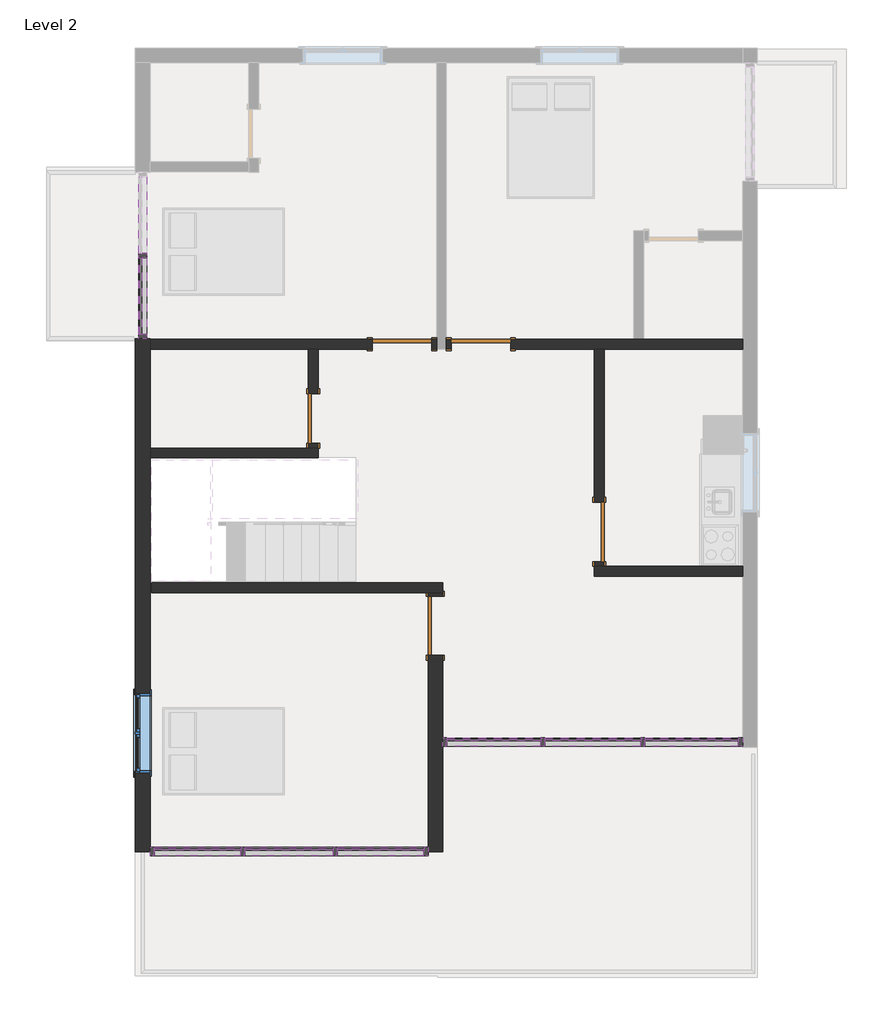
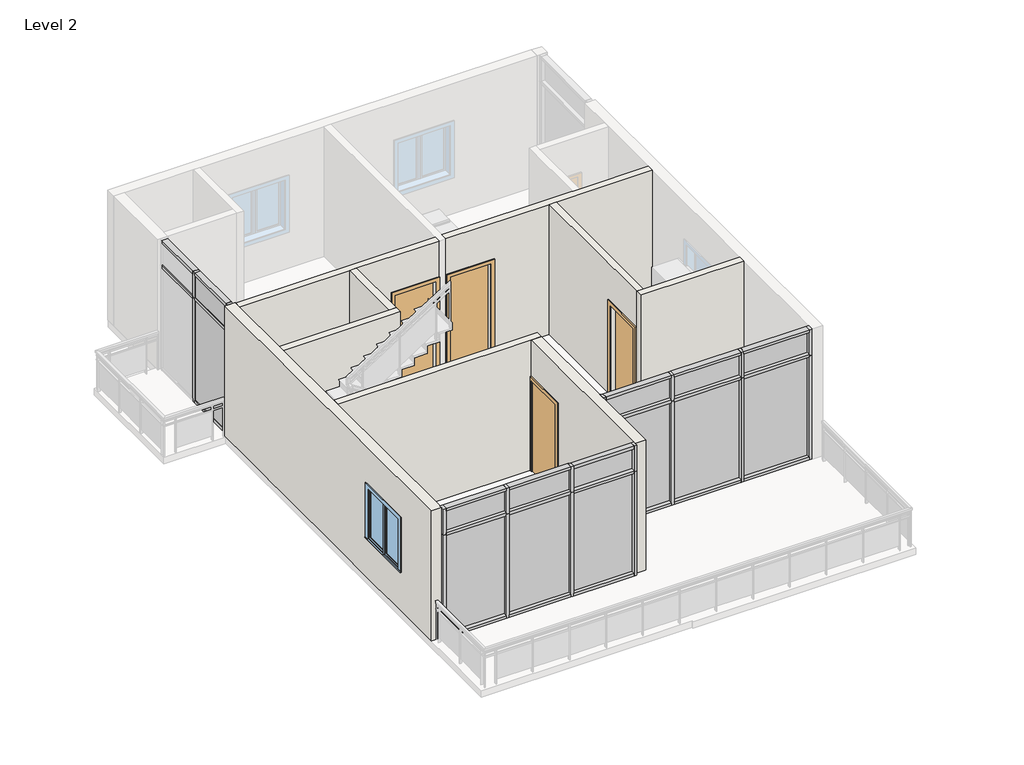
# One storey, part 1 of 3: 43 members, 14 plates, 9 walls, 5 doors, 1 window.
"""IFC4 building model written with IfcOpenShell, lengths in millimetres."""

from ifc_helpers import new_model, si_unit, frame, origin, place, context, project, spatial, polyline, outline, extrude, faceted_brep, transform, mapped, element, save
from components import single_flush_2_5_e2b13fe9, door_16372e1c, door_686f89d2, door_0ca8825f, member_ee409385, member_47bfaf8a, member_43f7a5f1, member_b3f2e294, member_f0fea5a5, member_6e77e263, member_77f995ea, member_70b51cdd, member_7a8c6f17, member_dbc9f771, member_0e93e1b1, member_1c68d6bd, member_709922c8, member_cd38fec7, system_panel_glazed_153bb9bb, system_panel_glazed_f2c52b8f, system_panel_glazed_8fc861e4, system_panel_glazed_97fa76a5, system_panel_glazed_70a1cf78, system_panel_glazed_f9c14314, system_panel_glazed_7a72b4ff, system_panel_glazed_660e552d, system_panel_glazed_652faff5, system_panel_glazed_2a82d765, window_8af0dca1

model = new_model("IFC4")

# Units and contexts
model_context = context("Model", 3, world=origin())
ifc_project = project(units=[si_unit("LENGTHUNIT", "METRE", prefix="MILLI")], contexts=[model_context])

# Site, building, storey
site = spatial("IfcSite", under=ifc_project)
building = spatial("IfcBuilding", under=site)
storey = spatial("IfcBuildingStorey", under=building, Name="Level 2", Elevation=3200.4)

# Doors
placement = place(None, origin())
single_flush_2_5_shape = single_flush_2_5_e2b13fe9(model_context)
element("IfcDoor", 1, ObjectType="Single-Flush : 2.5'", at=placement, inside=storey, context=model_context, shape_type="MappedRepresentation", body=[
    mapped(single_flush_2_5_shape, transform((-4970.2647018, 1970.8825188, 3200.4), x_axis=(0.0, -1.0, 0.0), y_axis=(1.0, 0.0, 0.0), z_axis=(0.0, 0.0, 1.0))),
])
door_shape = door_16372e1c(model_context)
element("IfcDoor", 2, ObjectType="Single-Flush : 36\" x 84\"", at=placement, inside=storey, context=model_context, shape_type="MappedRepresentation", body=[
    mapped(door_shape, transform((-3598.6647018, 3113.8825188, 3200.4), x_axis=(1.0, 0.0, 0.0), y_axis=(0.0, 1.0, 0.0), z_axis=(0.0, 0.0, 1.0))),
])
element("IfcDoor", 3, ObjectType="Single-Flush : 36\" x 84\"", at=placement, inside=storey, context=model_context, shape_type="MappedRepresentation", body=[
    mapped(door_shape, transform((-550.6647018, 218.2825188, 3200.4), x_axis=(0.0, -1.0, 0.0), y_axis=(1.0, 0.0, 0.0), z_axis=(0.0, 0.0, 1.0))),
])
door_2_shape = door_686f89d2(model_context)
element("IfcDoor", 4, ObjectType="Single-Flush : 36\" x 84\"", at=placement, inside=storey, context=model_context, shape_type="MappedRepresentation", body=[
    mapped(door_2_shape, transform((-2379.4647018, 3113.8825188, 3200.4), x_axis=(-1.0, 0.0, 0.0), y_axis=(0.0, -1.0, 0.0), z_axis=(0.0, 0.0, 1.0))),
])
door_3_shape = door_0ca8825f(model_context)
element("IfcDoor", 5, ObjectType="Single-Flush : 36\" x 84\"", at=placement, inside=storey, context=model_context, shape_type="MappedRepresentation", body=[
    mapped(door_3_shape, transform((-3081.8591614, -1228.9950563, 3200.4), x_axis=(0.0, 1.0, 0.0), y_axis=(-1.0, 0.0, 0.0), z_axis=(0.0, 0.0, 1.0))),
])

# Members
member_shape = member_ee409385(model_context)
element("IfcMember", 6, ObjectType="Rectangular Mullion : 2.5\" x 5\" rectangular", at=placement, inside=storey, context=model_context, shape_type="MappedRepresentation", body=[
    mapped(member_shape, transform((-3196.1591614, -4715.6674812, 3200.4), x_axis=(1.0, 0.0, 0.0), y_axis=(0.0, -1.0, 0.0), z_axis=(0.0, 0.0, -1.0))),
])
element("IfcMember", 7, ObjectType="Rectangular Mullion : 2.5\" x 5\" rectangular", at=placement, inside=storey, context=model_context, shape_type="MappedRepresentation", body=[
    mapped(member_shape, transform((-7484.8647018, -4715.6674812, 5638.8), x_axis=(-1.0, 0.0, 0.0), y_axis=(0.0, -1.0, 0.0), z_axis=(0.0, 0.0, 1.0))),
])
member_2_shape = member_47bfaf8a(model_context)
element("IfcMember", 8, ObjectType="Rectangular Mullion : 2.5\" x 5\" rectangular", at=placement, inside=storey, context=model_context, shape_type="MappedRepresentation", body=[
    mapped(member_2_shape, transform((-3196.1591614, -4715.6674812, 5638.8), x_axis=(1.0, 0.0, 0.0), y_axis=(0.0, -1.0, 0.0), z_axis=(0.0, 0.0, -1.0))),
])
element("IfcMember", 9, ObjectType="Rectangular Mullion : 2.5\" x 5\" rectangular", at=placement, inside=storey, context=model_context, shape_type="MappedRepresentation", body=[
    mapped(member_2_shape, transform((-7484.8647018, -4715.6674812, 6248.4), x_axis=(-1.0, 0.0, 0.0), y_axis=(0.0, -1.0, 0.0), z_axis=(0.0, 0.0, 1.0))),
])
member_3_shape = member_43f7a5f1(model_context)
element("IfcMember", 10, ObjectType="Rectangular Mullion : 2.5\" x 5\" rectangular", at=placement, inside=storey, context=model_context, shape_type="MappedRepresentation", body=[
    mapped(member_3_shape, transform((-7599.1647018, 3266.2825188, 6248.4), x_axis=(0.0, 0.0, 1.0), y_axis=(-1.0, 0.0, 0.0), z_axis=(0.0, -1.0, 0.0))),
])
element("IfcMember", 11, ObjectType="Rectangular Mullion : 2.5\" x 5\" rectangular", at=placement, inside=storey, context=model_context, shape_type="MappedRepresentation", body=[
    mapped(member_3_shape, transform((-7599.1647018, 4517.2325188, 6248.4), x_axis=(0.0, 0.0, 1.0), y_axis=(-1.0, 0.0, 0.0), z_axis=(0.0, -1.0, 0.0))),
])
element("IfcMember", 12, ObjectType="Rectangular Mullion : 2.5\" x 5\" rectangular", at=placement, inside=storey, context=model_context, shape_type="MappedRepresentation", body=[
    mapped(member_3_shape, transform((-7599.1647018, 4453.7325188, 3200.4), x_axis=(0.0, 0.0, -1.0), y_axis=(-1.0, 0.0, 0.0), z_axis=(0.0, 1.0, 0.0))),
])
member_4_shape = member_b3f2e294(model_context)
element("IfcMember", 13, ObjectType="Rectangular Mullion : 2.5\" x 5\" rectangular", at=placement, inside=storey, context=model_context, shape_type="MappedRepresentation", body=[
    mapped(member_4_shape, transform((-7599.1647018, 4517.2325188, 5638.8), x_axis=(0.0, 0.0, 1.0), y_axis=(-1.0, 0.0, 0.0), z_axis=(0.0, -1.0, 0.0))),
])
element("IfcMember", 14, ObjectType="Rectangular Mullion : 2.5\" x 5\" rectangular", at=placement, inside=storey, context=model_context, shape_type="MappedRepresentation", body=[
    mapped(member_4_shape, transform((-7599.1647018, 3266.2825188, 5638.8), x_axis=(0.0, 0.0, 1.0), y_axis=(-1.0, 0.0, 0.0), z_axis=(0.0, -1.0, 0.0))),
])
member_5_shape = member_f0fea5a5(model_context)
element("IfcMember", 15, ObjectType="Rectangular Mullion : 2.5\" x 5\" rectangular", at=placement, inside=storey, context=model_context, shape_type="MappedRepresentation", body=[
    mapped(member_5_shape, transform((-7599.1647018, 4485.4825188, 3200.4), x_axis=(0.0, -1.0, 0.0), y_axis=(-1.0, 0.0, 0.0), z_axis=(0.0, 0.0, -1.0))),
])
element("IfcMember", 16, ObjectType="Rectangular Mullion : 2.5\" x 5\" rectangular", at=placement, inside=storey, context=model_context, shape_type="MappedRepresentation", body=[
    mapped(member_5_shape, transform((116.9038116, -3026.0450563, 3200.4), x_axis=(-1.0, 0.0, 0.0), y_axis=(0.0, 1.0, 0.0), z_axis=(0.0, 0.0, -1.0))),
])
element("IfcMember", 17, ObjectType="Rectangular Mullion : 2.5\" x 5\" rectangular", at=placement, inside=storey, context=model_context, shape_type="MappedRepresentation", body=[
    mapped(member_5_shape, transform((-1425.3276749, -3026.0450563, 3200.4), x_axis=(-1.0, 0.0, 0.0), y_axis=(0.0, 1.0, 0.0), z_axis=(0.0, 0.0, -1.0))),
])
element("IfcMember", 18, ObjectType="Rectangular Mullion : 2.5\" x 5\" rectangular", at=placement, inside=storey, context=model_context, shape_type="MappedRepresentation", body=[
    mapped(member_shape, transform((-7599.1647018, 3202.7825188, 3200.4), x_axis=(0.0, -1.0, 0.0), y_axis=(-1.0, 0.0, 0.0), z_axis=(0.0, 0.0, -1.0))),
])
element("IfcMember", 19, ObjectType="Rectangular Mullion : 2.5\" x 5\" rectangular", at=placement, inside=storey, context=model_context, shape_type="MappedRepresentation", body=[
    mapped(member_shape, transform((-2967.5591614, -3026.0450563, 3200.4), x_axis=(-1.0, 0.0, 0.0), y_axis=(0.0, 1.0, 0.0), z_axis=(0.0, 0.0, -1.0))),
])
element("IfcMember", 20, ObjectType="Rectangular Mullion : 2.5\" x 5\" rectangular", at=placement, inside=storey, context=model_context, shape_type="MappedRepresentation", body=[
    mapped(member_shape, transform((1659.1352982, -3026.0450563, 5638.8), x_axis=(1.0, 0.0, 0.0), y_axis=(0.0, 1.0, 0.0), z_axis=(0.0, 0.0, 1.0))),
])
member_6_shape = member_6e77e263(model_context)
element("IfcMember", 21, ObjectType="Rectangular Mullion : 2.5\" x 5\" rectangular", at=placement, inside=storey, context=model_context, shape_type="MappedRepresentation", body=[
    mapped(member_6_shape, transform((-7599.1647018, 4485.4825188, 5638.8), x_axis=(0.0, -1.0, 0.0), y_axis=(-1.0, 0.0, 0.0), z_axis=(0.0, 0.0, -1.0))),
])
element("IfcMember", 22, ObjectType="Rectangular Mullion : 2.5\" x 5\" rectangular", at=placement, inside=storey, context=model_context, shape_type="MappedRepresentation", body=[
    mapped(member_6_shape, transform((116.9038116, -3026.0450563, 5638.8), x_axis=(-1.0, 0.0, 0.0), y_axis=(0.0, 1.0, 0.0), z_axis=(0.0, 0.0, -1.0))),
])
element("IfcMember", 23, ObjectType="Rectangular Mullion : 2.5\" x 5\" rectangular", at=placement, inside=storey, context=model_context, shape_type="MappedRepresentation", body=[
    mapped(member_6_shape, transform((-1425.3276749, -3026.0450563, 5638.8), x_axis=(-1.0, 0.0, 0.0), y_axis=(0.0, 1.0, 0.0), z_axis=(0.0, 0.0, -1.0))),
])
element("IfcMember", 24, ObjectType="Rectangular Mullion : 2.5\" x 5\" rectangular", at=placement, inside=storey, context=model_context, shape_type="MappedRepresentation", body=[
    mapped(member_2_shape, transform((-7599.1647018, 3202.7825188, 5638.8), x_axis=(0.0, -1.0, 0.0), y_axis=(-1.0, 0.0, 0.0), z_axis=(0.0, 0.0, -1.0))),
])
element("IfcMember", 25, ObjectType="Rectangular Mullion : 2.5\" x 5\" rectangular", at=placement, inside=storey, context=model_context, shape_type="MappedRepresentation", body=[
    mapped(member_2_shape, transform((-2967.5591614, -3026.0450563, 5638.8), x_axis=(-1.0, 0.0, 0.0), y_axis=(0.0, 1.0, 0.0), z_axis=(0.0, 0.0, -1.0))),
])
element("IfcMember", 26, ObjectType="Rectangular Mullion : 2.5\" x 5\" rectangular", at=placement, inside=storey, context=model_context, shape_type="MappedRepresentation", body=[
    mapped(member_2_shape, transform((1659.1352982, -3026.0450563, 6248.4), x_axis=(1.0, 0.0, 0.0), y_axis=(0.0, 1.0, 0.0), z_axis=(0.0, 0.0, 1.0))),
])
member_7_shape = member_77f995ea(model_context)
element("IfcMember", 27, ObjectType="Rectangular Mullion : 2.5\" x 5\" rectangular", at=placement, inside=storey, context=model_context, shape_type="MappedRepresentation", body=[
    mapped(member_7_shape, transform((-2904.0591614, -3026.0450563, 6248.4), x_axis=(0.0, 0.0, 1.0), y_axis=(0.0, 1.0, 0.0), z_axis=(-1.0, 0.0, 0.0))),
])
element("IfcMember", 28, ObjectType="Rectangular Mullion : 2.5\" x 5\" rectangular", at=placement, inside=storey, context=model_context, shape_type="MappedRepresentation", body=[
    mapped(member_7_shape, transform((148.6538116, -3026.0450563, 6248.4), x_axis=(0.0, 0.0, 1.0), y_axis=(0.0, 1.0, 0.0), z_axis=(-1.0, 0.0, 0.0))),
])
member_8_shape = member_70b51cdd(model_context)
element("IfcMember", 29, ObjectType="Rectangular Mullion : 2.5\" x 5\" rectangular", at=placement, inside=storey, context=model_context, shape_type="MappedRepresentation", body=[
    mapped(member_8_shape, transform((-1393.5776749, -3026.0450563, 6248.4), x_axis=(0.0, 0.0, 1.0), y_axis=(0.0, 1.0, 0.0), z_axis=(-1.0, 0.0, 0.0))),
])
element("IfcMember", 30, ObjectType="Rectangular Mullion : 2.5\" x 5\" rectangular", at=placement, inside=storey, context=model_context, shape_type="MappedRepresentation", body=[
    mapped(member_7_shape, transform((1595.6352982, -3026.0450563, 3200.4), x_axis=(0.0, 0.0, -1.0), y_axis=(0.0, 1.0, 0.0), z_axis=(1.0, 0.0, 0.0))),
])
element("IfcMember", 31, ObjectType="Rectangular Mullion : 2.5\" x 5\" rectangular", at=placement, inside=storey, context=model_context, shape_type="MappedRepresentation", body=[
    mapped(member_7_shape, transform((-1457.0776749, -3026.0450563, 3200.4), x_axis=(0.0, 0.0, -1.0), y_axis=(0.0, 1.0, 0.0), z_axis=(1.0, 0.0, 0.0))),
])
element("IfcMember", 32, ObjectType="Rectangular Mullion : 2.5\" x 5\" rectangular", at=placement, inside=storey, context=model_context, shape_type="MappedRepresentation", body=[
    mapped(member_8_shape, transform((85.1538116, -3026.0450563, 3200.4), x_axis=(0.0, 0.0, -1.0), y_axis=(0.0, 1.0, 0.0), z_axis=(1.0, 0.0, 0.0))),
])
member_9_shape = member_7a8c6f17(model_context)
element("IfcMember", 33, ObjectType="Rectangular Mullion : 2.5\" x 5\" rectangular", at=placement, inside=storey, context=model_context, shape_type="MappedRepresentation", body=[
    mapped(member_9_shape, transform((-1393.5776749, -3026.0450563, 5638.8), x_axis=(0.0, 0.0, 1.0), y_axis=(0.0, 1.0, 0.0), z_axis=(-1.0, 0.0, 0.0))),
])
member_10_shape = member_dbc9f771(model_context)
element("IfcMember", 34, ObjectType="Rectangular Mullion : 2.5\" x 5\" rectangular", at=placement, inside=storey, context=model_context, shape_type="MappedRepresentation", body=[
    mapped(member_10_shape, transform((-2904.0591614, -3026.0450563, 5638.8), x_axis=(0.0, 0.0, 1.0), y_axis=(0.0, 1.0, 0.0), z_axis=(-1.0, 0.0, 0.0))),
])
element("IfcMember", 35, ObjectType="Rectangular Mullion : 2.5\" x 5\" rectangular", at=placement, inside=storey, context=model_context, shape_type="MappedRepresentation", body=[
    mapped(member_10_shape, transform((148.6538116, -3026.0450563, 5638.8), x_axis=(0.0, 0.0, 1.0), y_axis=(0.0, 1.0, 0.0), z_axis=(-1.0, 0.0, 0.0))),
])
member_11_shape = member_0e93e1b1(model_context)
element("IfcMember", 36, ObjectType="Rectangular Mullion : 2.5\" x 5\" rectangular", at=placement, inside=storey, context=model_context, shape_type="MappedRepresentation", body=[
    mapped(member_11_shape, transform((-6023.5461884, -4715.6674812, 3200.4), x_axis=(0.0, 0.0, -1.0), y_axis=(0.0, -1.0, 0.0), z_axis=(-1.0, 0.0, 0.0))),
])
member_12_shape = member_1c68d6bd(model_context)
element("IfcMember", 37, ObjectType="Rectangular Mullion : 2.5\" x 5\" rectangular", at=placement, inside=storey, context=model_context, shape_type="MappedRepresentation", body=[
    mapped(member_12_shape, transform((-7421.3647018, -4715.6674812, 3200.4), x_axis=(0.0, 0.0, -1.0), y_axis=(0.0, -1.0, 0.0), z_axis=(-1.0, 0.0, 0.0))),
])
element("IfcMember", 38, ObjectType="Rectangular Mullion : 2.5\" x 5\" rectangular", at=placement, inside=storey, context=model_context, shape_type="MappedRepresentation", body=[
    mapped(member_12_shape, transform((-4593.9776749, -4715.6674812, 3200.4), x_axis=(0.0, 0.0, -1.0), y_axis=(0.0, -1.0, 0.0), z_axis=(-1.0, 0.0, 0.0))),
])
element("IfcMember", 39, ObjectType="Rectangular Mullion : 2.5\" x 5\" rectangular", at=placement, inside=storey, context=model_context, shape_type="MappedRepresentation", body=[
    mapped(member_12_shape, transform((-3259.6591614, -4715.6674812, 6248.4), x_axis=(0.0, 0.0, 1.0), y_axis=(0.0, -1.0, 0.0), z_axis=(1.0, 0.0, 0.0))),
])
element("IfcMember", 40, ObjectType="Rectangular Mullion : 2.5\" x 5\" rectangular", at=placement, inside=storey, context=model_context, shape_type="MappedRepresentation", body=[
    mapped(member_12_shape, transform((-6087.0461884, -4715.6674812, 6248.4), x_axis=(0.0, 0.0, 1.0), y_axis=(0.0, -1.0, 0.0), z_axis=(1.0, 0.0, 0.0))),
])
element("IfcMember", 41, ObjectType="Rectangular Mullion : 2.5\" x 5\" rectangular", at=placement, inside=storey, context=model_context, shape_type="MappedRepresentation", body=[
    mapped(member_11_shape, transform((-4657.4776749, -4715.6674812, 6248.4), x_axis=(0.0, 0.0, 1.0), y_axis=(0.0, -1.0, 0.0), z_axis=(1.0, 0.0, 0.0))),
])
element("IfcMember", 42, ObjectType="Rectangular Mullion : 2.5\" x 5\" rectangular", at=placement, inside=storey, context=model_context, shape_type="MappedRepresentation", body=[
    mapped(member_5_shape, transform((-6055.2961884, -4715.6674812, 3200.4), x_axis=(1.0, 0.0, 0.0), y_axis=(0.0, -1.0, 0.0), z_axis=(0.0, 0.0, -1.0))),
])
element("IfcMember", 43, ObjectType="Rectangular Mullion : 2.5\" x 5\" rectangular", at=placement, inside=storey, context=model_context, shape_type="MappedRepresentation", body=[
    mapped(member_5_shape, transform((-4625.7276749, -4715.6674812, 3200.4), x_axis=(1.0, 0.0, 0.0), y_axis=(0.0, -1.0, 0.0), z_axis=(0.0, 0.0, -1.0))),
])
member_13_shape = member_709922c8(model_context)
element("IfcMember", 44, ObjectType="Rectangular Mullion : 2.5\" x 5\" rectangular", at=placement, inside=storey, context=model_context, shape_type="MappedRepresentation", body=[
    mapped(member_13_shape, transform((-6087.0461884, -4715.6674812, 5638.8), x_axis=(0.0, 0.0, 1.0), y_axis=(0.0, -1.0, 0.0), z_axis=(1.0, 0.0, 0.0))),
])
element("IfcMember", 45, ObjectType="Rectangular Mullion : 2.5\" x 5\" rectangular", at=placement, inside=storey, context=model_context, shape_type="MappedRepresentation", body=[
    mapped(member_13_shape, transform((-3259.6591614, -4715.6674812, 5638.8), x_axis=(0.0, 0.0, 1.0), y_axis=(0.0, -1.0, 0.0), z_axis=(1.0, 0.0, 0.0))),
])
member_14_shape = member_cd38fec7(model_context)
element("IfcMember", 46, ObjectType="Rectangular Mullion : 2.5\" x 5\" rectangular", at=placement, inside=storey, context=model_context, shape_type="MappedRepresentation", body=[
    mapped(member_14_shape, transform((-4657.4776749, -4715.6674812, 5638.8), x_axis=(0.0, 0.0, 1.0), y_axis=(0.0, -1.0, 0.0), z_axis=(1.0, 0.0, 0.0))),
])
element("IfcMember", 47, ObjectType="Rectangular Mullion : 2.5\" x 5\" rectangular", at=placement, inside=storey, context=model_context, shape_type="MappedRepresentation", body=[
    mapped(member_6_shape, transform((-6055.2961884, -4715.6674812, 5638.8), x_axis=(1.0, 0.0, 0.0), y_axis=(0.0, -1.0, 0.0), z_axis=(0.0, 0.0, -1.0))),
])
element("IfcMember", 48, ObjectType="Rectangular Mullion : 2.5\" x 5\" rectangular", at=placement, inside=storey, context=model_context, shape_type="MappedRepresentation", body=[
    mapped(member_6_shape, transform((-4625.7276749, -4715.6674812, 5638.8), x_axis=(1.0, 0.0, 0.0), y_axis=(0.0, -1.0, 0.0), z_axis=(0.0, 0.0, -1.0))),
])

# Plates
system_panel_glazed_shape = system_panel_glazed_153bb9bb(model_context)
element("IfcPlate", 49, ObjectType="System Panel : Glazed", at=placement, inside=storey, context=model_context, shape_type="MappedRepresentation", body=[
    mapped(system_panel_glazed_shape, transform((-7599.1647018, 3860.0075188, 3263.9), x_axis=(0.0, -1.0, 0.0), y_axis=(1.0, 0.0, 0.0), z_axis=(0.0, 0.0, 1.0))),
])
system_panel_glazed_2_shape = system_panel_glazed_f2c52b8f(model_context)
element("IfcPlate", 50, ObjectType="System Panel : Glazed", at=placement, inside=storey, context=model_context, shape_type="MappedRepresentation", body=[
    mapped(system_panel_glazed_2_shape, transform((-7599.1647018, 3860.0075188, 5670.55), x_axis=(0.0, -1.0, 0.0), y_axis=(1.0, 0.0, 0.0), z_axis=(0.0, 0.0, 1.0))),
])
system_panel_glazed_3_shape = system_panel_glazed_8fc861e4(model_context)
element("IfcPlate", 51, ObjectType="System Panel : Glazed", at=placement, inside=storey, context=model_context, shape_type="MappedRepresentation", body=[
    mapped(system_panel_glazed_3_shape, transform((872.1445549, -3026.0450563, 3263.9), x_axis=(-1.0, 0.0, 0.0), y_axis=(0.0, -1.0, 0.0), z_axis=(0.0, 0.0, 1.0))),
])
element("IfcPlate", 52, ObjectType="System Panel : Glazed", at=placement, inside=storey, context=model_context, shape_type="MappedRepresentation", body=[
    mapped(system_panel_glazed_3_shape, transform((-2180.5684182, -3026.0450563, 3263.9), x_axis=(-1.0, 0.0, 0.0), y_axis=(0.0, -1.0, 0.0), z_axis=(0.0, 0.0, 1.0))),
])
system_panel_glazed_4_shape = system_panel_glazed_97fa76a5(model_context)
element("IfcPlate", 53, ObjectType="System Panel : Glazed", at=placement, inside=storey, context=model_context, shape_type="MappedRepresentation", body=[
    mapped(system_panel_glazed_4_shape, transform((-654.2119316, -3026.0450563, 3263.9), x_axis=(-1.0, 0.0, 0.0), y_axis=(0.0, -1.0, 0.0), z_axis=(0.0, 0.0, 1.0))),
])
system_panel_glazed_5_shape = system_panel_glazed_70a1cf78(model_context)
element("IfcPlate", 54, ObjectType="System Panel : Glazed", at=placement, inside=storey, context=model_context, shape_type="MappedRepresentation", body=[
    mapped(system_panel_glazed_5_shape, transform((872.1445549, -3026.0450563, 5670.55), x_axis=(-1.0, 0.0, 0.0), y_axis=(0.0, -1.0, 0.0), z_axis=(0.0, 0.0, 1.0))),
])
element("IfcPlate", 55, ObjectType="System Panel : Glazed", at=placement, inside=storey, context=model_context, shape_type="MappedRepresentation", body=[
    mapped(system_panel_glazed_5_shape, transform((-2180.5684182, -3026.0450563, 5670.55), x_axis=(-1.0, 0.0, 0.0), y_axis=(0.0, -1.0, 0.0), z_axis=(0.0, 0.0, 1.0))),
])
system_panel_glazed_6_shape = system_panel_glazed_f9c14314(model_context)
element("IfcPlate", 56, ObjectType="System Panel : Glazed", at=placement, inside=storey, context=model_context, shape_type="MappedRepresentation", body=[
    mapped(system_panel_glazed_6_shape, transform((-654.2119316, -3026.0450563, 5670.55), x_axis=(-1.0, 0.0, 0.0), y_axis=(0.0, -1.0, 0.0), z_axis=(0.0, 0.0, 1.0))),
])
system_panel_glazed_7_shape = system_panel_glazed_7a72b4ff(model_context)
element("IfcPlate", 57, ObjectType="System Panel : Glazed", at=placement, inside=storey, context=model_context, shape_type="MappedRepresentation", body=[
    mapped(system_panel_glazed_7_shape, transform((-6754.2054451, -4715.6674812, 3263.9), x_axis=(1.0, 0.0, 0.0), y_axis=(0.0, 1.0, 0.0), z_axis=(0.0, 0.0, 1.0))),
])
element("IfcPlate", 58, ObjectType="System Panel : Glazed", at=placement, inside=storey, context=model_context, shape_type="MappedRepresentation", body=[
    mapped(system_panel_glazed_7_shape, transform((-3926.8184182, -4715.6674812, 3263.9), x_axis=(1.0, 0.0, 0.0), y_axis=(0.0, 1.0, 0.0), z_axis=(0.0, 0.0, 1.0))),
])
system_panel_glazed_8_shape = system_panel_glazed_660e552d(model_context)
element("IfcPlate", 59, ObjectType="System Panel : Glazed", at=placement, inside=storey, context=model_context, shape_type="MappedRepresentation", body=[
    mapped(system_panel_glazed_8_shape, transform((-5340.5119316, -4715.6674812, 3263.9), x_axis=(1.0, 0.0, 0.0), y_axis=(0.0, 1.0, 0.0), z_axis=(0.0, 0.0, 1.0))),
])
system_panel_glazed_9_shape = system_panel_glazed_652faff5(model_context)
element("IfcPlate", 60, ObjectType="System Panel : Glazed", at=placement, inside=storey, context=model_context, shape_type="MappedRepresentation", body=[
    mapped(system_panel_glazed_9_shape, transform((-6754.2054451, -4715.6674812, 5670.55), x_axis=(1.0, 0.0, 0.0), y_axis=(0.0, 1.0, 0.0), z_axis=(0.0, 0.0, 1.0))),
])
element("IfcPlate", 61, ObjectType="System Panel : Glazed", at=placement, inside=storey, context=model_context, shape_type="MappedRepresentation", body=[
    mapped(system_panel_glazed_9_shape, transform((-3926.8184182, -4715.6674812, 5670.55), x_axis=(1.0, 0.0, 0.0), y_axis=(0.0, 1.0, 0.0), z_axis=(0.0, 0.0, 1.0))),
])
system_panel_glazed_10_shape = system_panel_glazed_2a82d765(model_context)
element("IfcPlate", 62, ObjectType="System Panel : Glazed", at=placement, inside=storey, context=model_context, shape_type="MappedRepresentation", body=[
    mapped(system_panel_glazed_10_shape, transform((-5340.5119316, -4715.6674812, 5670.55), x_axis=(1.0, 0.0, 0.0), y_axis=(0.0, 1.0, 0.0), z_axis=(0.0, 0.0, 1.0))),
])

# Walls
element("IfcWall", 63, ObjectType="6\"", at=placement, inside=storey, context=model_context, shape_type="Brep", body=[
    faceted_brep([(-3065.2647018, 3190.0825188, 3200.4), (-3141.4647018, 3190.0825188, 3200.4), (-3141.4647018, 3190.0825188, 5334.0), (-4055.8647018, 3190.0825188, 5334.0), (-4055.8647018, 3190.0825188, 3200.4), (-7484.8647018, 3190.0825188, 3200.4), (-7484.8647018, 3190.0825188, 6248.4), (-3065.2647018, 3190.0825188, 6248.4), (-3141.4647018, 3037.6825188, 5334.0), (-3141.4647018, 3037.6825188, 3200.4), (-3065.2647018, 3037.6825188, 3200.4), (-3065.2647018, 3037.6825188, 6248.4), (-4894.0647018, 3037.6825188, 6248.4), (-5046.4647018, 3037.6825188, 6248.4), (-7484.8647018, 3037.6825188, 6248.4), (-7484.8647018, 3037.6825188, 3200.4), (-5046.4647018, 3037.6825188, 3200.4), (-4894.0647018, 3037.6825188, 3200.4), (-4055.8647018, 3037.6825188, 3200.4), (-4055.8647018, 3037.6825188, 5334.0)], [[[0, 1, 2, 3, 4, 5, 6, 7]], [[8, 9, 10, 11, 12, 13, 14, 15, 16, 17, 18, 19]], [[10, 9, 1, 0]], [[18, 17, 16, 15, 5, 4]], [[7, 6, 14, 13, 12, 11]], [[0, 7, 11, 10]], [[6, 5, 15, 14]], [[2, 1, 9, 8]], [[3, 2, 8, 19]], [[4, 3, 19, 18]]]),
])
element("IfcWall", 64, ObjectType="6\"", at=placement, inside=storey, context=model_context, shape_type="Brep", body=[
    faceted_brep([(-2912.8647018, 3037.6825188, 3200.4), (-2836.6647018, 3037.6825188, 3200.4), (-2836.6647018, 3037.6825188, 5334.0), (-1922.2647018, 3037.6825188, 5334.0), (-1922.2647018, 3037.6825188, 3200.4), (-626.8647018, 3037.6825188, 3200.4), (-474.4647018, 3037.6825188, 3200.4), (1659.1352982, 3037.6825188, 3200.4), (1659.1352982, 3037.6825188, 6248.4), (-474.4647018, 3037.6825188, 6248.4), (-626.8647018, 3037.6825188, 6248.4), (-2912.8647018, 3037.6825188, 6248.4), (-2836.6647018, 3190.0825188, 5334.0), (-2836.6647018, 3190.0825188, 3200.4), (-2912.8647018, 3190.0825188, 3200.4), (-2912.8647018, 3190.0825188, 6248.4), (-17.2647018, 3190.0825188, 6248.4), (135.1352982, 3190.0825188, 6248.4), (1659.1352982, 3190.0825188, 6248.4), (1659.1352982, 3190.0825188, 3200.4), (135.1352982, 3190.0825188, 3200.4), (-17.2647018, 3190.0825188, 3200.4), (-1922.2647018, 3190.0825188, 3200.4), (-1922.2647018, 3190.0825188, 5334.0)], [[[0, 1, 2, 3, 4, 5, 6, 7, 8, 9, 10, 11]], [[12, 13, 14, 15, 16, 17, 18, 19, 20, 21, 22, 23]], [[14, 13, 1, 0]], [[22, 21, 20, 19, 7, 6, 5, 4]], [[11, 10, 9, 8, 18, 17, 16, 15]], [[0, 11, 15, 14]], [[8, 7, 19, 18]], [[2, 1, 13, 12]], [[3, 2, 12, 23]], [[4, 3, 23, 22]]]),
])
element("IfcWall", 65, ObjectType="6\"", at=placement, inside=storey, context=model_context, shape_type="Brep", body=[
    faceted_brep([(-7484.8647018, 1361.2825188, 3200.4), (-4894.0647018, 1361.2825188, 3200.4), (-4894.0647018, 1361.2825188, 6248.4), (-7484.8647018, 1361.2825188, 6248.4), (-7484.8647018, 1513.6825188, 3200.4), (-7484.8647018, 1513.6825188, 6248.4), (-5046.4647018, 1513.6825188, 6248.4), (-4894.0647018, 1513.6825188, 6248.4), (-4894.0647018, 1513.6825188, 3200.4), (-5046.4647018, 1513.6825188, 3200.4)], [[[0, 1, 2, 3]], [[4, 5, 6, 7, 8, 9]], [[1, 0, 4, 9, 8]], [[3, 2, 7, 6, 5]], [[0, 3, 5, 4]], [[2, 1, 8, 7]]]),
])
element("IfcWall", 66, ObjectType="6\"", at=placement, inside=storey, context=model_context, shape_type="SweptSolid", body=[
    extrude(outline(polyline([(1589.8825188, 5334.0), (1589.8825188, 3200.4), (1513.6825188, 3200.4), (1513.6825188, 6248.4), (3037.6825188, 6248.4), (3037.6825188, 3200.4), (2351.8825188, 3200.4), (2351.8825188, 5334.0), (1589.8825188, 5334.0)])), frame((-5046.4647018, 0.0, 0.0), z_axis=(1.0, 0.0, 0.0), x_axis=(0.0, 1.0, 0.0)), (0.0, 0.0, 1.0), 152.4),
])
element("IfcWall", 67, ObjectType="6\"", at=placement, inside=storey, context=model_context, shape_type="Brep", body=[
    faceted_brep([(1659.1352982, -315.1174812, 3200.4), (-474.4647018, -315.1174812, 3200.4), (-626.8647018, -315.1174812, 3200.4), (-626.8647018, -315.1174812, 6248.4), (-474.4647018, -315.1174812, 6248.4), (1659.1352982, -315.1174812, 6248.4), (1659.1352982, -467.5174812, 3200.4), (1659.1352982, -467.5174812, 6248.4), (-626.8647018, -467.5174812, 6248.4), (-626.8647018, -467.5174812, 3200.4)], [[[0, 1, 2, 3, 4, 5]], [[6, 7, 8, 9]], [[2, 1, 0, 6, 9]], [[5, 4, 3, 8, 7]], [[0, 5, 7, 6]], [[3, 2, 9, 8]]]),
])
element("IfcWall", 68, ObjectType="6\"", at=placement, inside=storey, context=model_context, shape_type="SweptSolid", body=[
    extrude(outline(polyline([(-238.9174812, 5334.0), (-238.9174812, 3200.4), (-315.1174812, 3200.4), (-315.1174812, 6248.4), (3037.6825188, 6248.4), (3037.6825188, 3200.4), (675.4825188, 3200.4), (675.4825188, 5334.0), (-238.9174812, 5334.0)])), frame((-626.8647018, 0.0, 0.0), z_axis=(1.0, 0.0, 0.0), x_axis=(0.0, 1.0, 0.0)), (0.0, 0.0, 1.0), 152.4),
])
element("IfcWall", 69, ObjectType="6\"", at=placement, inside=storey, context=model_context, shape_type="Brep", body=[
    faceted_brep([(-7463.3591614, -720.9950563, 3200.4), (-3196.1591614, -720.9950563, 3200.4), (-2967.5591614, -720.9950563, 3200.4), (-2967.5591614, -720.9950563, 6248.4), (-3196.1591614, -720.9950563, 6248.4), (-7463.3591614, -720.9950563, 6248.4), (-7463.3591614, -568.5950563, 3200.4), (-7463.3591614, -568.5950563, 6248.4), (-2967.5591614, -568.5950563, 6248.4), (-2967.5591614, -568.5950563, 3200.4)], [[[0, 1, 2, 3, 4, 5]], [[6, 7, 8, 9]], [[2, 1, 0, 6, 9]], [[5, 4, 3, 8, 7]], [[0, 5, 7, 6]], [[3, 2, 9, 8]]]),
])
element("IfcWall", 70, ObjectType="9\"", at=placement, inside=storey, context=model_context, shape_type="SweptSolid", body=[
    extrude(outline(polyline([(-720.9950563, 3200.4), (-771.7950563, 3200.4), (-771.7950563, 5334.0), (-1686.1950563, 5334.0), (-1686.1950563, 3200.4), (-4715.6674812, 3200.4), (-4715.6674812, 6248.4), (-720.9950563, 6248.4), (-720.9950563, 3200.4)])), frame((-3196.1591614, 0.0, 0.0), z_axis=(1.0, 0.0, 0.0), x_axis=(0.0, 1.0, 0.0)), (0.0, 0.0, 1.0), 228.6),
])
element("IfcWall", 71, ObjectType="9\"", at=placement, inside=storey, context=model_context, shape_type="Brep", body=[
    faceted_brep([(-7713.4647018, 3202.7825188, 3200.4), (-7713.4647018, -4715.6674812, 3200.4), (-7713.4647018, -4715.6674812, 6248.4), (-7713.4647018, 3202.7825188, 6248.4), (-7713.4647018, -2277.2674812, 5334.0), (-7713.4647018, -3496.4674812, 5334.0), (-7713.4647018, -3496.4674812, 4114.8), (-7713.4647018, -2277.2674812, 4114.8), (-7484.8647018, 3202.7825188, 3200.4), (-7484.8647018, 3202.7825188, 6248.4), (-7484.8647018, 3190.0825188, 6248.4), (-7484.8647018, 3037.6825188, 6248.4), (-7484.8647018, 1513.6825188, 6248.4), (-7484.8647018, 1361.2825188, 6248.4), (-7484.8647018, -4715.6674812, 6248.4), (-7484.8647018, -4715.6674812, 3200.4), (-7484.8647018, 1361.2825188, 3200.4), (-7484.8647018, 1513.6825188, 3200.4), (-7484.8647018, 3037.6825188, 3200.4), (-7484.8647018, 3190.0825188, 3200.4), (-7484.8647018, -2277.2674812, 5334.0), (-7484.8647018, -2277.2674812, 4114.8), (-7484.8647018, -3496.4674812, 4114.8), (-7484.8647018, -3496.4674812, 5334.0)], [[[0, 1, 2, 3], [4, 5, 6, 7]], [[8, 9, 10, 11, 12, 13, 14, 15, 16, 17, 18, 19], [20, 21, 22, 23]], [[1, 0, 8, 19, 18, 17, 16, 15]], [[2, 1, 15, 14]], [[3, 2, 14, 13, 12, 11, 10, 9]], [[0, 3, 9, 8]], [[21, 20, 4, 7]], [[22, 21, 7, 6]], [[23, 22, 6, 5]], [[20, 23, 5, 4]]]),
])

# Window
window_shape = window_8af0dca1(model_context)
element("IfcWindow", 72, ObjectType="Casement Dbl with Trim : 48\" x 48\"", at=placement, inside=storey, context=model_context, shape_type="MappedRepresentation", body=[
    mapped(window_shape, transform((-7580.1147018, -2886.8674812, 3352.8), x_axis=(0.0, 1.0, 0.0), y_axis=(-1.0, 0.0, 0.0), z_axis=(0.0, 0.0, 1.0))),
])

save(model, "model.ifc")

# Revit data of these elements
# Type "Single-Flush : 2.5'"
#   Type Mark = "8"
#   Construction Type Id = "MDOOR"
#   Assembly Code = "C1020"
#   Analytic Construction = "Metal"
#   Thickness = 0' - 2"
#   Heat Transfer Coefficient (U) = 0.651978 BTU/(h·ft²·°F)
#   Height = 7' - 0"
#   Trim Projection Ext = 0' - 1"
#   Trim Projection Int = 0' - 1"
#   Trim Width = 0' - 3"
#   Width = 2' - 6"
#   Define Thermal Properties by = 1
#   Door Material = Door - Panel
#   Frame Material = Door - Frame
#   Visual Light Transmittance = 0
#   Solar Heat Gain Coefficient = 0
#   Function = (empty or 0)
#   Wall Closure = (empty or 0)
# Type "Single-Flush : 36\" x 84\""
#   Type Mark = "1"
#   Construction Type Id = "MDOOR"
#   Assembly Code = "C1020"
#   Analytic Construction = "Metal"
#   Thickness = 0' - 2"
#   Heat Transfer Coefficient (U) = 0.651978 BTU/(h·ft²·°F)
#   Height = 7' - 0"
#   Trim Projection Ext = 0' - 1"
#   Trim Projection Int = 0' - 1"
#   Trim Width = 0' - 3"
#   Width = 3' - 0"
#   Define Thermal Properties by = 1
#   Door Material = Door - Panel
#   Frame Material = Door - Frame
#   Visual Light Transmittance = 0
#   Solar Heat Gain Coefficient = 0
#   Function = (empty or 0)
#   Wall Closure = (empty or 0)
# Type "Rectangular Mullion : 2.5\" x 5\" rectangular"
#   built-in parameter 1007304 = 0.416667 (stored number, unit not read)
#   built-in parameter 1007301 = 0.104167 (stored number, unit not read)
#   built-in parameter 1007300 = 0.104167 (stored number, unit not read)
# Type "System Panel : Glazed"
#   Construction Type Id = "GSP4R"
#   Analytic Construction = "1/8 in Pilkington single glazing"
#   Visual Light Transmittance = 0.9
#   Solar Heat Gain Coefficient = 0.86
#   Heat Transfer Coefficient (U) = 1.18115 BTU/(h·ft²·°F)
# Type "6\""
#   Assembly Code = "B2010"
#   Layers, outside or top first: 0' - 6" "inner wall" (function 1)
# Type "9\""
#   Assembly Code = "B2010"
#   Layers, outside or top first: 0' - 9" "ext wall" (function 1)
# Type "Casement Dbl with Trim : 48\" x 48\""
#   Type Mark = "10"
#   Construction Type Id = "GSP4R"
#   Assembly Code = "B2020100"
#   Analytic Construction = "1/8 in Pilkington single glazing"
#   Visual Light Transmittance = 0.9
#   Solar Heat Gain Coefficient = 0.78
#   Heat Transfer Coefficient (U) = 0.6496 BTU/(h·ft²·°F)
#   Height = 4' - 0"
#   Default Sill Height = 2' - 6"
#   Trim Projection - Ext. = 0' - 0 1/2"
#   Trim Projection - Int. = 0' - 0 3/4"
#   Trim Width - Exterior = 0' - 3 1/2"
#   Trim Width - Interior = 0' - 3 1/2"
#   Width = 4' - 0"
#   Window Inset = 0' - 0 3/4"
#   Define Thermal Properties by = 1
#   Glass Pane Material = Glass
#   Sash Material = Sash
#   Trim Exterior Material = Trim
#   Trim Interior Material = Trim
#   Wall Closure = (empty or 0)
# Element 1 (IfcDoor, "Single-Flush : 2.5'")
#   Phase Created = New Construction
#   Materials on its faces: "Door - Frame", "Door - Panel"
# Elements 2, 3, 4, 5 (IfcDoor, "Single-Flush : 36\" x 84\"")
#   Phase Created = New Construction
#   Materials on its faces: "Door - Frame", "Door - Panel"
# Elements 6, 7, 8, 9, 10, 11, 12, 13, 14, 15, 16, 17, 18, 19, 20, 21, 22, 23, 24, 25, 26, 27, 28, 29, 30, 31, 32, 33, 34, 35, 36, 37, 38, 39, 40, 41, 42, 43, 44, 45, 46, 47, 48 (IfcMember, "Rectangular Mullion : 2.5\" x 5\" rectangular")
#   Phase Created = New Construction
#   Materials on its faces: "Aluminum"
# Elements 49, 50, 51, 52, 53, 54, 55, 56, 57, 58, 59, 60, 61, 62 (IfcPlate, "System Panel : Glazed")
#   Phase Created = New Construction
#   Materials on its faces: "Glass"
# Elements 63, 64, 65, 66, 67, 68 (IfcWall, "6\"")
#   Top Offset = 0' - 0"
#   Base Offset = 0' - 0"
#   Unconnected Height = 10' - 0"
#   wall height = 10' - 0"
#   Phase Created = New Construction
#   Base Constraint = Level 2
#   Materials on its faces: "inner wall"
# Element 69 (IfcWall, "6\"")
#   Top Offset = 0' - 0"
#   Base Offset = 0' - 0"
#   Unconnected Height = 10' - 0"
#   wall height = 10' - 0"
#   Phase Created = New Construction
#   Base Constraint = Level 2
#   Materials on its faces: "inner wall", "ext wall"
# Elements 70, 71 (IfcWall, "9\"")
#   Top Offset = 0' - 0"
#   Base Offset = 0' - 0"
#   Unconnected Height = 10' - 0"
#   wall height = 10' - 0"
#   Phase Created = New Construction
#   Base Constraint = Level 2
#   Materials on its faces: "ext wall", "inner wall"
# Element 72 (IfcWindow, "Casement Dbl with Trim : 48\" x 48\"")
#   Mark = "9"
#   Phase Created = New Construction
#   Materials on its faces: "Sash", "Trim", "Glass"
# Materials
#   "Door - Panel": class "Wood", colour RGB 210 159 95, transparency 0
#   "Door - Frame": colour RGB 118 70 51, transparency 0
#   "inner wall": class "Generic", colour RGB 230 213 172, transparency 0, Cost = 0
#   "ext wall": class "Generic", colour RGB 153 153 153, transparency 0, Cost = 0
#   "Glass": class "Glass", colour RGB 0 128 192, transparency 0.75, Description = "Soda Lime Glass", Cost = 0
#   "Sash": class "Wood", colour RGB 224 178 126, transparency 0
#   "Trim": class "Wood", colour RGB 224 178 126, transparency 0
#   "Aluminum": class "Metal", colour RGB 247 247 247, transparency 0, Description = "Aluminum 6061", Cost = 0
